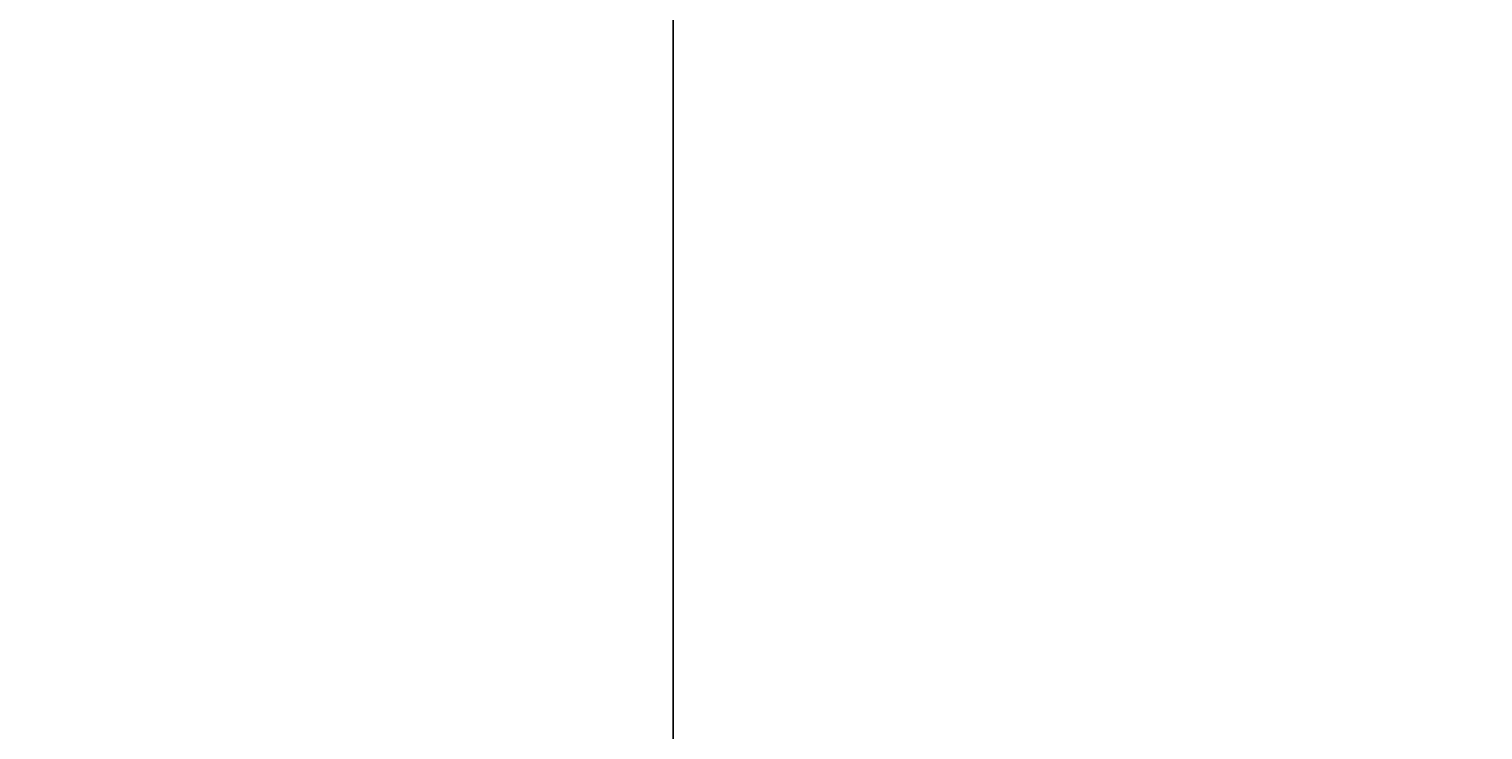
# Model space of a CAD drawing. Units: inches. Extents: x -61 to 1599, y -1316 to 257.
# Tile 109 of 204: x 200 to 236, y -135 to -117. Entities that reach past the tile are written whole.
import ezdxf

# ---------------------------------------------------------------- set-up
doc = ezdxf.new("R2010")
doc.units = ezdxf.units.IN
doc.header["$MEASUREMENT"] = 0
doc.layers.add('A-ANNO-DIMS', color=2, linetype='Continuous', lineweight=18)
doc.styles.get("Standard").update_dxf_attribs({"font": 'arial.ttf'})
doc.dimstyles.get("Standard").update_dxf_attribs({"dimtxt": 0.18, "dimasz": 0.18, "dimexe": 0.18, "dimexo": 0.0625, "dimgap": 0.09, "dimtad": 0, "dimtih": 1, "dimtoh": 1, "dimdec": 0, "dimzin": 0, "dimdsep": 46, "dimlunit": 3, "dimtxsty": 'Standard', "dimcen": 0.09, "dimadec": 0, "dimazin": 0, "dimtfac": 1, "dimtdec": 0, "dimtofl": 0, "dimtmove": 0, "dimatfit": 3, "dimfxl": 1, "dimtolj": 1, "dimtzin": 0, "dimarcsym": 0})

# ---------------------------------------------------------------- blocks, each defined once
blk = doc.blocks.new('*D687')
at = {"layer": 'A-ANNO-DIMS', "color": 0, "lineweight": -2, "transparency": 16777216}
for p, q in [((289.418, 181.677), (-61.077, 181.677)), ((-60.897, 181.497), (-60.897, -528.952)), ((-60.897, -1239.765), (-60.897, -529.316)), ((319.64, -1239.945), (-61.077, -1239.945))]:
    blk.add_line(p, q, dxfattribs=at)
at = {"layer": 'A-ANNO-DIMS', "color": 0, "transparency": 16777216}
for points in [[(-60.927, 181.497), (-60.867, 181.497), (-60.897, 181.677)], [(-60.927, -1239.765), (-60.867, -1239.765), (-60.897, -1239.945)]]:
    blk.add_solid(points, dxfattribs=at)
at = {"layer": 'DEFPOINTS', "color": 0, "transparency": 16777216}
for p in [(289.481, 181.677), (-60.897, -1239.945), (319.703, -1239.945)]:
    blk.add_point(p, dxfattribs=at)
at = {"layer": 'A-ANNO-DIMS', "color": 0, "transparency": 16777216, "insert": (-60.897, -529.134), "char_height": 0.18, "attachment_point": 5}
blk.add_mtext('\\A1;1421.6', dxfattribs=at)
blk = doc.blocks.new('*D701')
at = {"layer": 'A-ANNO-DIMS', "color": 0, "lineweight": -2, "transparency": 16777216}
for p, q in [((215.752, -616.882), (215.752, 257.457)), ((252.882, -616.882), (252.882, 257.457)), ((215.932, 257.277), (233.924, 257.277)), ((252.702, 257.277), (234.711, 257.277))]:
    blk.add_line(p, q, dxfattribs=at)
at = {"layer": 'A-ANNO-DIMS', "color": 0, "transparency": 16777216}
for points in [[(215.932, 257.307), (215.932, 257.247), (215.752, 257.277)], [(252.702, 257.307), (252.702, 257.247), (252.882, 257.277)]]:
    blk.add_solid(points, dxfattribs=at)
at = {"layer": 'DEFPOINTS', "color": 0, "transparency": 16777216}
for p in [(252.882, 257.277), (215.752, -616.945), (252.882, -616.945)]:
    blk.add_point(p, dxfattribs=at)
at = {"layer": 'A-ANNO-DIMS', "color": 0, "transparency": 16777216, "insert": (234.317, 257.277), "char_height": 0.18, "attachment_point": 5}
blk.add_mtext('\\A1;37.13', dxfattribs=at)

msp = doc.modelspace()

# ---------------------------------------------------------------- dimensions: what is measured, and where the dimension line sits
at = {"layer": 'A-ANNO-DIMS'}
dim = msp.add_linear_dim(base=(252.8825, 257.2771), p1=(215.7521, -616.9446), p2=(252.8825, -616.9446), dimstyle='Standard', override={"dimdec": 2, "dimlfac": 1, "dimrnd": 0, "dimzin": 0, "dimdsep": 46, "dimlunit": 2}, dxfattribs=at)
dim.commit()
dim.dimension.update_dxf_attribs({"geometry": '*D701', "text_midpoint": (234.3173, 257.2771)})
dim = msp.add_linear_dim(base=(-60.8972, -1239.9446), p1=(289.4807, 181.6771), p2=(319.7028, -1239.9446), angle=90, dimstyle='Standard', override={"dimdec": 1, "dimlfac": 1, "dimrnd": 0, "dimzin": 0, "dimdsep": 46, "dimlunit": 2}, dxfattribs=at)
dim.commit()
dim.dimension.update_dxf_attribs({"geometry": '*D687', "text_midpoint": (-60.8972, -529.1337)})

doc.saveas('drawing.dxf')
